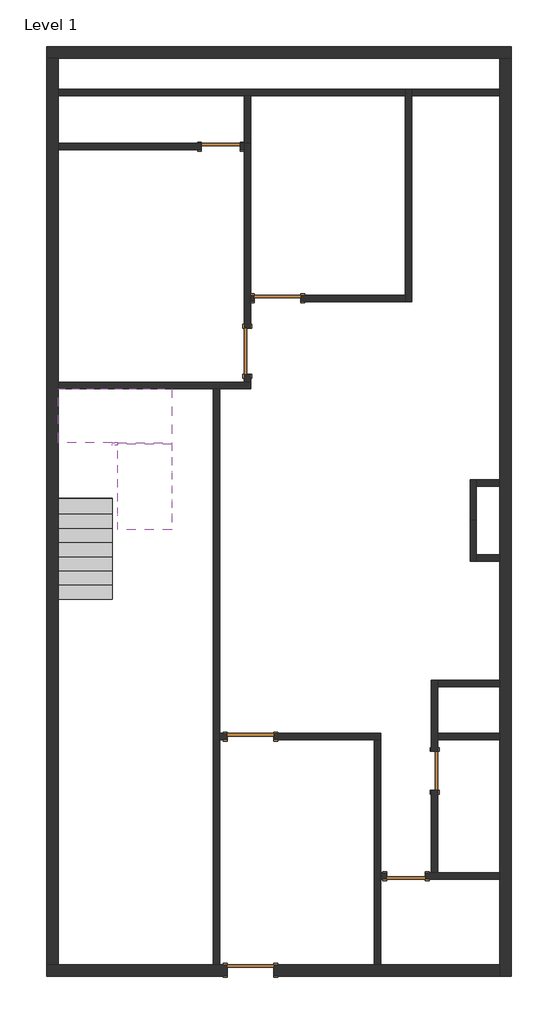
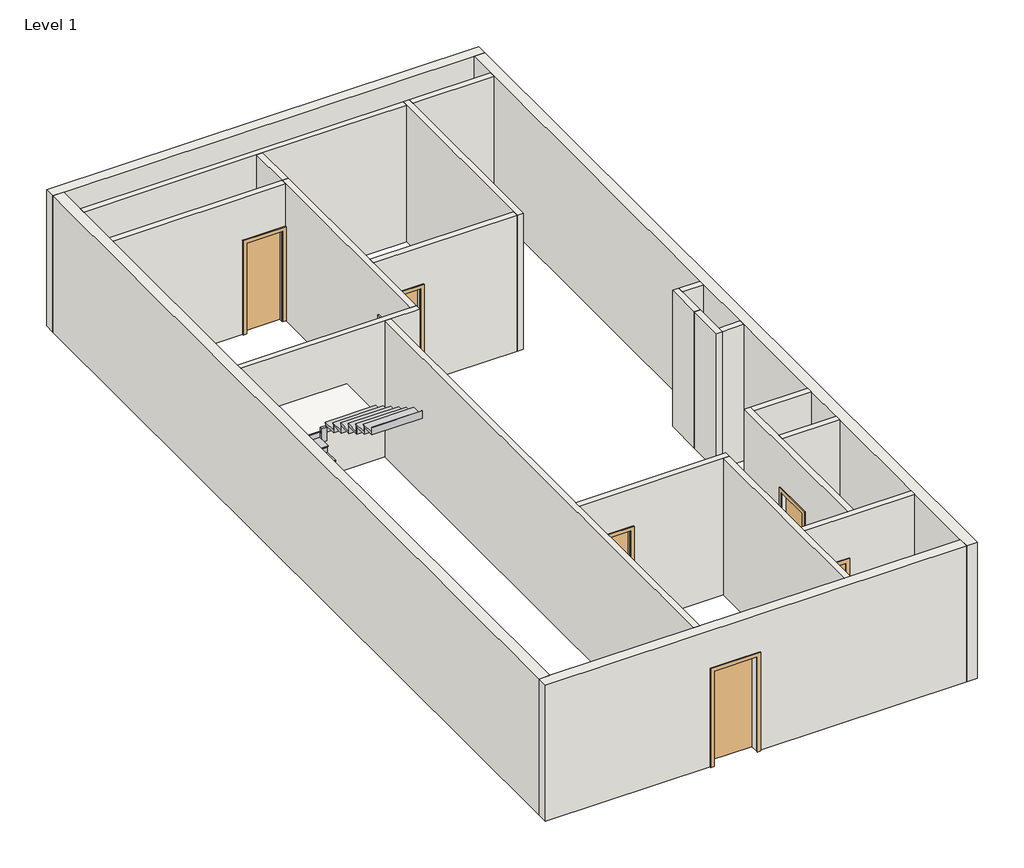
# One storey: 23 walls, 7 doors, 2 stair flights, 1 member, 1 slab.
"""IFC4 building model written with IfcOpenShell, lengths in millimetres."""

from ifc_helpers import new_model, si_unit, frame, origin, origin_with_axes, place, context, project, spatial, polyline, outline, extrude, faceted_brep, transform, mapped, element, save
from components import door_1fe7f57d, door_e00f436c, door_a3eb833a, door_a90ba1ad, non_monolithic_landing_dd6d84fa, stair_flight_4c38af94, stair_flight_924b7841

model = new_model("IFC4")

# Units and contexts
model_context = context("Model", 3, world=origin())
ifc_project = project(units=[si_unit("LENGTHUNIT", "METRE", prefix="MILLI")], contexts=[model_context])

# Site, building, storey
site = spatial("IfcSite", under=ifc_project)
building = spatial("IfcBuilding", under=site)
storey = spatial("IfcBuildingStorey", under=building, Name="Level 1", Elevation=0.0)

# Doors
placement = place(None, origin())
door_shape = door_1fe7f57d(model_context)
element("IfcDoor", 1, ObjectType="Single-Flush : 30\" x 80\"", at=placement, inside=storey, context=model_context, shape_type="MappedRepresentation", body=[
    mapped(door_shape, transform((592.3661131, -3666.3531144, 0.0), x_axis=(-1.0, 0.0, 0.0), y_axis=(0.0, -1.0, 0.0), z_axis=(0.0, 0.0, 1.0))),
])
element("IfcDoor", 2, ObjectType="Single-Flush : 30\" x 80\"", at=placement, inside=storey, context=model_context, shape_type="MappedRepresentation", body=[
    mapped(door_shape, transform((-3052.5338869, 10684.6468856, 0.0), x_axis=(1.0, 0.0, 0.0), y_axis=(0.0, 1.0, 0.0), z_axis=(0.0, 0.0, 1.0))),
])
door_2_shape = door_e00f436c(model_context)
element("IfcDoor", 3, ObjectType="Single-Flush : 30\" x 80\"", at=placement, inside=storey, context=model_context, shape_type="MappedRepresentation", body=[
    mapped(door_2_shape, transform((1151.1661131, -1596.2531144, 0.0), x_axis=(0.0, 1.0, 0.0), y_axis=(-1.0, 0.0, 0.0), z_axis=(0.0, 0.0, 1.0))),
])
door_3_shape = door_a3eb833a(model_context)
element("IfcDoor", 4, ObjectType="Single-Flush : 36\" x 84\"", at=placement, inside=storey, context=model_context, shape_type="MappedRepresentation", body=[
    mapped(door_3_shape, transform((-2531.8338869, 6658.7468856, 0.0), x_axis=(0.0, -1.0, 0.0), y_axis=(1.0, 0.0, 0.0), z_axis=(0.0, 0.0, 1.0))),
])
element("IfcDoor", 5, ObjectType="Single-Flush : 36\" x 84\"", at=placement, inside=storey, context=model_context, shape_type="MappedRepresentation", body=[
    mapped(door_3_shape, transform((-1934.9338869, 7700.1468856, 0.0), x_axis=(-1.0, 0.0, 0.0), y_axis=(0.0, -1.0, 0.0), z_axis=(0.0, 0.0, 1.0))),
])
element("IfcDoor", 6, ObjectType="Single-Flush : 36\" x 84\"", at=placement, inside=storey, context=model_context, shape_type="MappedRepresentation", body=[
    mapped(door_3_shape, transform((-2468.3338869, -923.1531144, 0.0), x_axis=(-1.0, 0.0, 0.0), y_axis=(0.0, -1.0, 0.0), z_axis=(0.0, 0.0, 1.0))),
])
door_4_shape = door_a90ba1ad(model_context)
element("IfcDoor", 7, ObjectType="Single-Flush : 36\" x 84\"", at=placement, inside=storey, context=model_context, shape_type="MappedRepresentation", body=[
    mapped(door_4_shape, transform((-2468.3338869, -5520.5531144, 0.0), x_axis=(-1.0, 0.0, 0.0), y_axis=(0.0, -1.0, 0.0), z_axis=(0.0, 0.0, 1.0))),
])

# Member
element("IfcMember", 8, ObjectType="Stringer - 2\" Width", at=placement, inside=storey, context=model_context, shape_type="SweptSolid", body=[
    extrude(outline(polyline([(-5186.1338869, 4804.5468856), (-5186.1338869, 4855.3468856), (-5084.5338869, 4855.3468856), (-5084.5338869, 4804.5468856), (-5186.1338869, 4804.5468856)])), frame((0.0, 0.0, 1696.4526316), z_axis=(0.0, 0.0, 1.0), x_axis=(1.0, 0.0, 0.0)), (0.0, 0.0, 1.0), 304.8),
])

# Slab
non_monolithic_landing_shape = non_monolithic_landing_dd6d84fa(model_context)
element("IfcSlab", 9, ObjectType="Non-Monolithic Landing", at=placement, inside=storey, context=model_context, shape_type="MappedRepresentation", body=[
    mapped(non_monolithic_landing_shape, transform((0.0, 0.0, 0.0), x_axis=(1.0, 0.0, 0.0), y_axis=(0.0, 1.0, 0.0), z_axis=(0.0, 0.0, 1.0))),
])

# Stair flights
stair_flight_shape = stair_flight_4c38af94(model_context)
element("IfcStairFlight", 10, ObjectType="2\" Tread 1\" Nosing 1/4\" Riser", at=placement, inside=storey, context=model_context, shape_type="MappedRepresentation", body=[
    mapped(stair_flight_shape, transform((0.0, 0.0, 0.0), x_axis=(1.0, 0.0, 0.0), y_axis=(0.0, 1.0, 0.0), z_axis=(0.0, 0.0, 1.0))),
])
stair_flight_2_shape = stair_flight_924b7841(model_context)
element("IfcStairFlight", 11, ObjectType="2\" Tread 1\" Nosing 1/4\" Riser", at=placement, inside=storey, context=model_context, shape_type="MappedRepresentation", body=[
    mapped(stair_flight_2_shape, transform((0.0, 0.0, 0.0), x_axis=(1.0, 0.0, 0.0), y_axis=(0.0, 1.0, 0.0), z_axis=(0.0, 0.0, 1.0))),
])

# Walls
element("IfcWall", 12, ObjectType="Generic - 5\"", at=placement, inside=storey, context=model_context, shape_type="Brep", body=[
    faceted_brep([(-6252.9338869, 5922.1468856, 0.0), (-3204.9338869, 5922.1468856, 0.0), (-3077.9338869, 5922.1468856, 0.0), (-2468.3338869, 5922.1468856, 0.0), (-2468.3338869, 5922.1468856, 3048.0), (-3077.9338869, 5922.1468856, 3048.0), (-3204.9338869, 5922.1468856, 3048.0), (-6252.9338869, 5922.1468856, 3048.0), (-6252.9338869, 6049.1468856, 0.0), (-6252.9338869, 6049.1468856, 3048.0), (-2595.3338869, 6049.1468856, 3048.0), (-2468.3338869, 6049.1468856, 3048.0), (-2468.3338869, 6049.1468856, 0.0), (-2595.3338869, 6049.1468856, 0.0)], [[[0, 1, 2, 3, 4, 5, 6, 7]], [[8, 9, 10, 11, 12, 13]], [[3, 2, 1, 0, 8, 13, 12]], [[7, 6, 5, 4, 11, 10, 9]], [[0, 7, 9, 8]], [[4, 3, 12, 11]]]),
])
element("IfcWall", 13, ObjectType="Generic - 5\"", at=placement, inside=storey, context=model_context, shape_type="Brep", body=[
    faceted_brep([(-3204.9338869, 5922.1468856, 0.0), (-3204.9338869, -5406.2531144, 0.0), (-3204.9338869, -5406.2531144, 3048.0), (-3204.9338869, 5922.1468856, 3048.0), (-3077.9338869, 5922.1468856, 0.0), (-3077.9338869, 5922.1468856, 3048.0), (-3077.9338869, -859.6531144, 3048.0), (-3077.9338869, -986.6531144, 3048.0), (-3077.9338869, -5406.2531144, 3048.0), (-3077.9338869, -5406.2531144, 0.0), (-3077.9338869, -986.6531144, 0.0), (-3077.9338869, -859.6531144, 0.0)], [[[0, 1, 2, 3]], [[4, 5, 6, 7, 8, 9, 10, 11]], [[1, 0, 4, 11, 10, 9]], [[3, 2, 8, 7, 6, 5]], [[0, 3, 5, 4]], [[2, 1, 9, 8]]]),
])
element("IfcWall", 14, ObjectType="Generic - 5\"", at=placement, inside=storey, context=model_context, shape_type="Brep", body=[
    faceted_brep([(-2925.5338869, -859.6531144, 2133.6), (-2925.5338869, -859.6531144, 0.0), (-3077.9338869, -859.6531144, 0.0), (-3077.9338869, -859.6531144, 3048.0), (97.0661131, -859.6531144, 3048.0), (97.0661131, -859.6531144, 0.0), (-2011.1338869, -859.6531144, 0.0), (-2011.1338869, -859.6531144, 2133.6), (-3077.9338869, -986.6531144, 0.0), (-2925.5338869, -986.6531144, 0.0), (-2925.5338869, -986.6531144, 2133.6), (-2011.1338869, -986.6531144, 2133.6), (-2011.1338869, -986.6531144, 0.0), (-29.9338869, -986.6531144, 0.0), (97.0661131, -986.6531144, 0.0), (97.0661131, -986.6531144, 3048.0), (-29.9338869, -986.6531144, 3048.0), (-3077.9338869, -986.6531144, 3048.0)], [[[0, 1, 2, 3, 4, 5, 6, 7]], [[8, 9, 10, 11, 12, 13, 14, 15, 16, 17]], [[6, 5, 14, 13, 12]], [[2, 1, 9, 8]], [[4, 3, 17, 16, 15]], [[5, 4, 15, 14]], [[3, 2, 8, 17]], [[10, 9, 1, 0]], [[11, 10, 0, 7]], [[12, 11, 7, 6]]]),
])
element("IfcWall", 15, ObjectType="Generic - 5\"", at=placement, inside=storey, context=model_context, shape_type="Brep", body=[
    faceted_brep([(-2468.3338869, 6049.1468856, 0.0), (-2468.3338869, 6201.5468856, 0.0), (-2468.3338869, 6201.5468856, 2133.6), (-2468.3338869, 7115.9468856, 2133.6), (-2468.3338869, 7115.9468856, 0.0), (-2468.3338869, 7636.6468856, 0.0), (-2468.3338869, 7763.6468856, 0.0), (-2468.3338869, 10748.1468856, 0.0), (-2468.3338869, 10748.1468856, 3048.0), (-2468.3338869, 7763.6468856, 3048.0), (-2468.3338869, 7636.6468856, 3048.0), (-2468.3338869, 6049.1468856, 3048.0), (-2595.3338869, 6201.5468856, 2133.6), (-2595.3338869, 6201.5468856, 0.0), (-2595.3338869, 6049.1468856, 0.0), (-2595.3338869, 6049.1468856, 3048.0), (-2595.3338869, 10621.1468856, 3048.0), (-2595.3338869, 10748.1468856, 3048.0), (-2595.3338869, 10748.1468856, 0.0), (-2595.3338869, 10621.1468856, 0.0), (-2595.3338869, 7115.9468856, 0.0), (-2595.3338869, 7115.9468856, 2133.6)], [[[0, 1, 2, 3, 4, 5, 6, 7, 8, 9, 10, 11]], [[12, 13, 14, 15, 16, 17, 18, 19, 20, 21]], [[14, 13, 1, 0]], [[20, 19, 18, 7, 6, 5, 4]], [[11, 10, 9, 8, 17, 16, 15]], [[8, 7, 18, 17]], [[0, 11, 15, 14]], [[2, 1, 13, 12]], [[3, 2, 12, 21]], [[4, 3, 21, 20]]]),
])
element("IfcWall", 16, ObjectType="Generic - 5\"", at=placement, inside=storey, context=model_context, shape_type="SweptSolid", body=[
    extrude(outline(polyline([(2032.0, -2671.5338869), (0.0, -2671.5338869), (0.0, -2595.3338869), (3048.0, -2595.3338869), (3048.0, -6252.9338869), (0.0, -6252.9338869), (0.0, -3433.5338869), (2032.0, -3433.5338869), (2032.0, -2671.5338869)])), frame((0.0, 10621.1468856, 0.0), z_axis=(0.0, 1.0, 0.0), x_axis=(0.0, 0.0, 1.0)), (0.0, 0.0, 1.0), 127.0),
])
element("IfcWall", 17, ObjectType="Generic - 5\"", at=placement, inside=storey, context=model_context, shape_type="SweptSolid", body=[
    extrude(outline(polyline([(-2468.3338869, 11687.9468856), (-2468.3338869, 10748.1468856), (-2595.3338869, 10748.1468856), (-2595.3338869, 11687.9468856), (-2468.3338869, 11687.9468856)])), origin_with_axes(), (0.0, 0.0, 1.0), 3048.0),
])
element("IfcWall", 18, ObjectType="Generic - 5\"", at=placement, inside=storey, context=model_context, shape_type="Brep", body=[
    faceted_brep([(579.6661131, 11814.9468856, 0.0), (-6252.9338869, 11814.9468856, 0.0), (-6252.9338869, 11814.9468856, 3048.0), (579.6661131, 11814.9468856, 3048.0), (579.6661131, 11687.9468856, 0.0), (579.6661131, 11687.9468856, 3048.0), (-2468.3338869, 11687.9468856, 3048.0), (-2595.3338869, 11687.9468856, 3048.0), (-6252.9338869, 11687.9468856, 3048.0), (-6252.9338869, 11687.9468856, 0.0), (-2595.3338869, 11687.9468856, 0.0), (-2468.3338869, 11687.9468856, 0.0)], [[[0, 1, 2, 3]], [[4, 5, 6, 7, 8, 9, 10, 11]], [[1, 0, 4, 11, 10, 9]], [[3, 2, 8, 7, 6, 5]], [[2, 1, 9, 8]], [[0, 3, 5, 4]]]),
])
element("IfcWall", 19, ObjectType="Generic - 5\"", at=placement, inside=storey, context=model_context, shape_type="Brep", body=[
    faceted_brep([(579.6661131, 11814.9468856, 0.0), (579.6661131, 11687.9468856, 0.0), (579.6661131, 7763.6468856, 0.0), (579.6661131, 7636.6468856, 0.0), (579.6661131, 7636.6468856, 3048.0), (579.6661131, 7763.6468856, 3048.0), (579.6661131, 11687.9468856, 3048.0), (579.6661131, 11814.9468856, 3048.0), (706.6661131, 11814.9468856, 0.0), (706.6661131, 11814.9468856, 3048.0), (706.6661131, 11687.9468856, 3048.0), (706.6661131, 7636.6468856, 3048.0), (706.6661131, 7636.6468856, 0.0), (706.6661131, 11687.9468856, 0.0)], [[[0, 1, 2, 3, 4, 5, 6, 7]], [[8, 9, 10, 11, 12, 13]], [[3, 2, 1, 0, 8, 13, 12]], [[7, 6, 5, 4, 11, 10, 9]], [[0, 7, 9, 8]], [[4, 3, 12, 11]]]),
])
element("IfcWall", 20, ObjectType="Generic - 5\"", at=placement, inside=storey, context=model_context, shape_type="SweptSolid", body=[
    extrude(outline(polyline([(2433.8661131, 11687.9468856), (706.6661131, 11687.9468856), (706.6661131, 11814.9468856), (2433.8661131, 11814.9468856), (2433.8661131, 11687.9468856)])), origin_with_axes(), (0.0, 0.0, 1.0), 3048.0),
])
element("IfcWall", 21, ObjectType="Generic - 5\"", at=placement, inside=storey, context=model_context, shape_type="SweptSolid", body=[
    extrude(outline(polyline([(0.0, -2468.3338869), (0.0, -2392.1338869), (2133.6, -2392.1338869), (2133.6, -1477.7338869), (0.0, -1477.7338869), (0.0, 579.6661131), (3048.0, 579.6661131), (3048.0, -2468.3338869), (0.0, -2468.3338869)])), frame((0.0, 7636.6468856, 0.0), z_axis=(0.0, 1.0, 0.0), x_axis=(0.0, 0.0, 1.0)), (0.0, 0.0, 1.0), 127.0),
])
element("IfcWall", 22, ObjectType="Generic - 5\"", at=placement, inside=storey, context=model_context, shape_type="Brep", body=[
    faceted_brep([(-29.9338869, -986.6531144, 0.0), (-29.9338869, -5406.2531144, 0.0), (-29.9338869, -5406.2531144, 3048.0), (-29.9338869, -986.6531144, 3048.0), (97.0661131, -986.6531144, 0.0), (97.0661131, -986.6531144, 3048.0), (97.0661131, -3602.8531144, 3048.0), (97.0661131, -3729.8531144, 3048.0), (97.0661131, -5406.2531144, 3048.0), (97.0661131, -5406.2531144, 0.0), (97.0661131, -3729.8531144, 0.0), (97.0661131, -3602.8531144, 0.0)], [[[0, 1, 2, 3]], [[4, 5, 6, 7, 8, 9, 10, 11]], [[1, 0, 4, 11, 10, 9]], [[3, 2, 8, 7, 6, 5]], [[2, 1, 9, 8]], [[0, 3, 5, 4]]]),
])
element("IfcWall", 23, ObjectType="Generic - 5\"", at=placement, inside=storey, context=model_context, shape_type="Brep", body=[
    faceted_brep([(97.0661131, -3729.8531144, 0.0), (211.3661131, -3729.8531144, 0.0), (211.3661131, -3729.8531144, 2032.0), (973.3661131, -3729.8531144, 2032.0), (973.3661131, -3729.8531144, 0.0), (2433.8661131, -3729.8531144, 0.0), (2433.8661131, -3729.8531144, 3048.0), (97.0661131, -3729.8531144, 3048.0), (211.3661131, -3602.8531144, 2032.0), (211.3661131, -3602.8531144, 0.0), (97.0661131, -3602.8531144, 0.0), (97.0661131, -3602.8531144, 3048.0), (1087.6661131, -3602.8531144, 3048.0), (1214.6661131, -3602.8531144, 3048.0), (2433.8661131, -3602.8531144, 3048.0), (2433.8661131, -3602.8531144, 0.0), (1214.6661131, -3602.8531144, 0.0), (1087.6661131, -3602.8531144, 0.0), (973.3661131, -3602.8531144, 0.0), (973.3661131, -3602.8531144, 2032.0)], [[[0, 1, 2, 3, 4, 5, 6, 7]], [[8, 9, 10, 11, 12, 13, 14, 15, 16, 17, 18, 19]], [[10, 9, 1, 0]], [[18, 17, 16, 15, 5, 4]], [[7, 6, 14, 13, 12, 11]], [[6, 5, 15, 14]], [[0, 7, 11, 10]], [[2, 1, 9, 8]], [[3, 2, 8, 19]], [[4, 3, 19, 18]]]),
])
element("IfcWall", 24, ObjectType="Generic - 5\"", at=placement, inside=storey, context=model_context, shape_type="Brep", body=[
    faceted_brep([(1214.6661131, -1215.2531144, 2032.0), (1214.6661131, -1215.2531144, 0.0), (1214.6661131, -986.6531144, 0.0), (1214.6661131, -859.6531144, 0.0), (1214.6661131, 54.7468856, 0.0), (1214.6661131, 181.7468856, 0.0), (1214.6661131, 181.7468856, 3048.0), (1214.6661131, 54.7468856, 3048.0), (1214.6661131, -859.6531144, 3048.0), (1214.6661131, -986.6531144, 3048.0), (1214.6661131, -3602.8531144, 3048.0), (1214.6661131, -3602.8531144, 0.0), (1214.6661131, -1977.2531144, 0.0), (1214.6661131, -1977.2531144, 2032.0), (1087.6661131, 181.7468856, 0.0), (1087.6661131, -1215.2531144, 0.0), (1087.6661131, -1215.2531144, 2032.0), (1087.6661131, -1977.2531144, 2032.0), (1087.6661131, -1977.2531144, 0.0), (1087.6661131, -3602.8531144, 0.0), (1087.6661131, -3602.8531144, 3048.0), (1087.6661131, 181.7468856, 3048.0)], [[[0, 1, 2, 3, 4, 5, 6, 7, 8, 9, 10, 11, 12, 13]], [[14, 15, 16, 17, 18, 19, 20, 21]], [[12, 11, 19, 18]], [[5, 4, 3, 2, 1, 15, 14]], [[10, 9, 8, 7, 6, 21, 20]], [[11, 10, 20, 19]], [[6, 5, 14, 21]], [[16, 15, 1, 0]], [[17, 16, 0, 13]], [[18, 17, 13, 12]]]),
])
element("IfcWall", 25, ObjectType="Generic - 5\"", at=placement, inside=storey, context=model_context, shape_type="SweptSolid", body=[
    extrude(outline(polyline([(2433.8661131, -986.6531144), (1214.6661131, -986.6531144), (1214.6661131, -859.6531144), (2433.8661131, -859.6531144), (2433.8661131, -986.6531144)])), origin_with_axes(), (0.0, 0.0, 1.0), 3048.0),
])
element("IfcWall", 26, ObjectType="Generic - 5\"", at=placement, inside=storey, context=model_context, shape_type="SweptSolid", body=[
    extrude(outline(polyline([(2433.8661131, 54.7468856), (1214.6661131, 54.7468856), (1214.6661131, 181.7468856), (2433.8661131, 181.7468856), (2433.8661131, 54.7468856)])), origin_with_axes(), (0.0, 0.0, 1.0), 3048.0),
])
element("IfcWall", 27, ObjectType="Generic - 5\"", at=placement, inside=storey, context=model_context, shape_type="Brep", body=[
    faceted_brep([(1976.6661131, 3331.3468856, 0.0), (1976.6661131, 4004.4468856, 0.0), (1976.6661131, 4131.4468856, 0.0), (1976.6661131, 4131.4468856, 3048.0), (1976.6661131, 4004.4468856, 3048.0), (1976.6661131, 3331.3468856, 3048.0), (1849.6661131, 3331.3468856, 0.0), (1849.6661131, 3331.3468856, 3048.0), (1849.6661131, 4131.4468856, 3048.0), (1849.6661131, 4131.4468856, 0.0)], [[[0, 1, 2, 3, 4, 5]], [[6, 7, 8, 9]], [[2, 1, 0, 6, 9]], [[5, 4, 3, 8, 7]], [[0, 5, 7, 6]], [[3, 2, 9, 8]]]),
])
element("IfcWall", 28, ObjectType="Generic - 5\"", at=placement, inside=storey, context=model_context, shape_type="SweptSolid", body=[
    extrude(outline(polyline([(2433.8661131, 4004.4468856), (1976.6661131, 4004.4468856), (1976.6661131, 4131.4468856), (2433.8661131, 4131.4468856), (2433.8661131, 4004.4468856)])), origin_with_axes(), (0.0, 0.0, 1.0), 3048.0),
])
element("IfcWall", 29, ObjectType="Generic - 5\"", at=placement, inside=storey, context=model_context, shape_type="Brep", body=[
    faceted_brep([(1849.6661131, 3331.3468856, 0.0), (1849.6661131, 2531.2468856, 0.0), (1849.6661131, 2531.2468856, 3048.0), (1849.6661131, 3331.3468856, 3048.0), (1976.6661131, 3331.3468856, 0.0), (1976.6661131, 3331.3468856, 3048.0), (1976.6661131, 2658.2468856, 3048.0), (1976.6661131, 2531.2468856, 3048.0), (1976.6661131, 2531.2468856, 0.0), (1976.6661131, 2658.2468856, 0.0)], [[[0, 1, 2, 3]], [[4, 5, 6, 7, 8, 9]], [[1, 0, 4, 9, 8]], [[3, 2, 7, 6, 5]], [[0, 3, 5, 4]], [[2, 1, 8, 7]]]),
])
element("IfcWall", 30, ObjectType="Generic - 5\"", at=placement, inside=storey, context=model_context, shape_type="SweptSolid", body=[
    extrude(outline(polyline([(2433.8661131, 2531.2468856), (1976.6661131, 2531.2468856), (1976.6661131, 2658.2468856), (2433.8661131, 2658.2468856), (2433.8661131, 2531.2468856)])), origin_with_axes(), (0.0, 0.0, 1.0), 3048.0),
])
element("IfcWall", 31, ObjectType="Generic - 9\"", at=placement, inside=storey, context=model_context, shape_type="Brep", body=[
    faceted_brep([(-6481.5338869, 12424.5468856, 0.0), (-6252.9338869, 12424.5468856, 0.0), (2433.8661131, 12424.5468856, 0.0), (2662.4661131, 12424.5468856, 0.0), (2662.4661131, 12424.5468856, 3048.0), (2433.8661131, 12424.5468856, 3048.0), (-6252.9338869, 12424.5468856, 3048.0), (-6481.5338869, 12424.5468856, 3048.0), (-6481.5338869, 12653.1468856, 0.0), (-6481.5338869, 12653.1468856, 3048.0), (2662.4661131, 12653.1468856, 3048.0), (2662.4661131, 12653.1468856, 0.0)], [[[0, 1, 2, 3, 4, 5, 6, 7]], [[8, 9, 10, 11]], [[3, 2, 1, 0, 8, 11]], [[7, 6, 5, 4, 10, 9]], [[4, 3, 11, 10]], [[0, 7, 9, 8]]]),
])
element("IfcWall", 32, ObjectType="Generic - 9\"", at=placement, inside=storey, context=model_context, shape_type="Brep", body=[
    faceted_brep([(2433.8661131, 12424.5468856, 0.0), (2433.8661131, 11814.9468856, 0.0), (2433.8661131, 11687.9468856, 0.0), (2433.8661131, 4131.4468856, 0.0), (2433.8661131, 4004.4468856, 0.0), (2433.8661131, 2658.2468856, 0.0), (2433.8661131, 2531.2468856, 0.0), (2433.8661131, 181.7468856, 0.0), (2433.8661131, 54.7468856, 0.0), (2433.8661131, -859.6531144, 0.0), (2433.8661131, -986.6531144, 0.0), (2433.8661131, -3602.8531144, 0.0), (2433.8661131, -3729.8531144, 0.0), (2433.8661131, -5406.2531144, 0.0), (2433.8661131, -5634.8531144, 0.0), (2433.8661131, -5634.8531144, 3048.0), (2433.8661131, -5406.2531144, 3048.0), (2433.8661131, -3729.8531144, 3048.0), (2433.8661131, -3602.8531144, 3048.0), (2433.8661131, -986.6531144, 3048.0), (2433.8661131, -859.6531144, 3048.0), (2433.8661131, 54.7468856, 3048.0), (2433.8661131, 181.7468856, 3048.0), (2433.8661131, 2531.2468856, 3048.0), (2433.8661131, 2658.2468856, 3048.0), (2433.8661131, 4004.4468856, 3048.0), (2433.8661131, 4131.4468856, 3048.0), (2433.8661131, 11687.9468856, 3048.0), (2433.8661131, 11814.9468856, 3048.0), (2433.8661131, 12424.5468856, 3048.0), (2662.4661131, 12424.5468856, 0.0), (2662.4661131, 12424.5468856, 3048.0), (2662.4661131, -5634.8531144, 3048.0), (2662.4661131, -5634.8531144, 0.0)], [[[0, 1, 2, 3, 4, 5, 6, 7, 8, 9, 10, 11, 12, 13, 14, 15, 16, 17, 18, 19, 20, 21, 22, 23, 24, 25, 26, 27, 28, 29]], [[30, 31, 32, 33]], [[14, 13, 12, 11, 10, 9, 8, 7, 6, 5, 4, 3, 2, 1, 0, 30, 33]], [[29, 28, 27, 26, 25, 24, 23, 22, 21, 20, 19, 18, 17, 16, 15, 32, 31]], [[0, 29, 31, 30]], [[15, 14, 33, 32]]]),
])
element("IfcWall", 33, ObjectType="Generic - 9\"", at=placement, inside=storey, context=model_context, shape_type="Brep", body=[
    faceted_brep([(-2925.5338869, -5406.2531144, 2133.6), (-2925.5338869, -5406.2531144, 0.0), (-3077.9338869, -5406.2531144, 0.0), (-3204.9338869, -5406.2531144, 0.0), (-6252.9338869, -5406.2531144, 0.0), (-6481.5338869, -5406.2531144, 0.0), (-6481.5338869, -5406.2531144, 3048.0), (-6252.9338869, -5406.2531144, 3048.0), (-3204.9338869, -5406.2531144, 3048.0), (-3077.9338869, -5406.2531144, 3048.0), (-29.9338869, -5406.2531144, 3048.0), (97.0661131, -5406.2531144, 3048.0), (2433.8661131, -5406.2531144, 3048.0), (2433.8661131, -5406.2531144, 0.0), (97.0661131, -5406.2531144, 0.0), (-29.9338869, -5406.2531144, 0.0), (-2011.1338869, -5406.2531144, 0.0), (-2011.1338869, -5406.2531144, 2133.6), (-6481.5338869, -5634.8531144, 0.0), (-2925.5338869, -5634.8531144, 0.0), (-2925.5338869, -5634.8531144, 2133.6), (-2011.1338869, -5634.8531144, 2133.6), (-2011.1338869, -5634.8531144, 0.0), (2433.8661131, -5634.8531144, 0.0), (2433.8661131, -5634.8531144, 3048.0), (-6481.5338869, -5634.8531144, 3048.0)], [[[0, 1, 2, 3, 4, 5, 6, 7, 8, 9, 10, 11, 12, 13, 14, 15, 16, 17]], [[18, 19, 20, 21, 22, 23, 24, 25]], [[5, 4, 3, 2, 1, 19, 18]], [[16, 15, 14, 13, 23, 22]], [[12, 11, 10, 9, 8, 7, 6, 25, 24]], [[13, 12, 24, 23]], [[6, 5, 18, 25]], [[20, 19, 1, 0]], [[21, 20, 0, 17]], [[22, 21, 17, 16]]]),
])
element("IfcWall", 34, ObjectType="Generic - 9\"", at=placement, inside=storey, context=model_context, shape_type="Brep", body=[
    faceted_brep([(-6252.9338869, -5406.2531144, 0.0), (-6252.9338869, 5922.1468856, 0.0), (-6252.9338869, 6049.1468856, 0.0), (-6252.9338869, 10621.1468856, 0.0), (-6252.9338869, 10748.1468856, 0.0), (-6252.9338869, 11687.9468856, 0.0), (-6252.9338869, 11814.9468856, 0.0), (-6252.9338869, 12424.5468856, 0.0), (-6252.9338869, 12424.5468856, 3048.0), (-6252.9338869, 11814.9468856, 3048.0), (-6252.9338869, 11687.9468856, 3048.0), (-6252.9338869, 10748.1468856, 3048.0), (-6252.9338869, 10621.1468856, 3048.0), (-6252.9338869, 6049.1468856, 3048.0), (-6252.9338869, 5922.1468856, 3048.0), (-6252.9338869, -5406.2531144, 3048.0), (-6481.5338869, -5406.2531144, 0.0), (-6481.5338869, -5406.2531144, 3048.0), (-6481.5338869, 12424.5468856, 3048.0), (-6481.5338869, 12424.5468856, 0.0)], [[[0, 1, 2, 3, 4, 5, 6, 7, 8, 9, 10, 11, 12, 13, 14, 15]], [[16, 17, 18, 19]], [[7, 6, 5, 4, 3, 2, 1, 0, 16, 19]], [[15, 14, 13, 12, 11, 10, 9, 8, 18, 17]], [[8, 7, 19, 18]], [[0, 15, 17, 16]]]),
])

save(model, "model.ifc")

# Revit data of these elements
# Type "Single-Flush : 30\" x 80\""
#   Type Mark = "5"
#   Assembly Code = "C1020"
#   Thickness = 0' - 2"
#   Height = 6' - 8"
#   Trim Projection Ext = 0' - 1"
#   Trim Projection Int = 0' - 1"
#   Trim Width = 0' - 3"
#   Width = 2' - 6"
#   Door Material = Door - Panel
#   Frame Material = Door - Frame
#   Function = (empty or 0)
#   Wall Closure = (empty or 0)
# Type "Single-Flush : 36\" x 84\""
#   Type Mark = "1"
#   Assembly Code = "C1020"
#   Thickness = 0' - 2"
#   Height = 7' - 0"
#   Trim Projection Ext = 0' - 1"
#   Trim Projection Int = 0' - 1"
#   Trim Width = 0' - 3"
#   Width = 3' - 0"
#   Door Material = Door - Panel
#   Frame Material = Door - Frame
#   Function = (empty or 0)
#   Wall Closure = (empty or 0)
# Type "Generic - 5\""
#   Assembly Code = "B2010"
#   Layers, outside or top first: 0' - 5" no material (function 1)
# Type "Generic - 9\""
#   Assembly Code = "B2010"
#   Layers, outside or top first: 0' - 9" no material (function 1)
# Elements 1, 2, 3 (IfcDoor, "Single-Flush : 30\" x 80\"")
#   Phase Created = New Construction
#   Materials on its faces: "Door - Frame", "Door - Panel"
# Elements 4, 5, 6, 7 (IfcDoor, "Single-Flush : 36\" x 84\"")
#   Phase Created = New Construction
#   Materials on its faces: "Door - Frame", "Door - Panel"
# Element 8 (IfcMember, "Stringer - 2\" Width")
#   Phase Created = New Construction
# Element 9 (IfcSlab, "Non-Monolithic Landing")
#   Phase Created = New Construction
# Elements 10, 11 (IfcStairFlight, "2\" Tread 1\" Nosing 1/4\" Riser")
#   Phase Created = New Construction
# Elements 12, 13, 14, 15, 16, 17, 18, 19, 20, 21, 22, 23, 24, 25, 26, 27, 28, 29, 30 (IfcWall, "Generic - 5\"")
#   Top Offset = 0' - 0"
#   Base Offset = 0' - 0"
#   Unconnected Height = 10' - 0"
#   wall height = 10' - 0"
#   Phase Created = New Construction
#   Base Constraint = Level 1
#   Materials on its faces: "Default Wall"
# Elements 31, 32, 33, 34 (IfcWall, "Generic - 9\"")
#   Top Offset = 0' - 0"
#   Base Offset = 0' - 0"
#   Unconnected Height = 10' - 0"
#   wall height = 10' - 0"
#   Phase Created = New Construction
#   Base Constraint = Level 1
#   Materials on its faces: "Default Wall"
# Materials
#   "Door - Panel": class "Wood", colour RGB 114 82 51, transparency 0
#   "Door - Frame": colour RGB 153 76 43, transparency 0
#   "Default Wall": colour RGB 80 80 80, transparency 0
